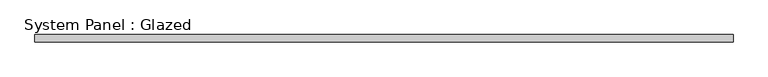
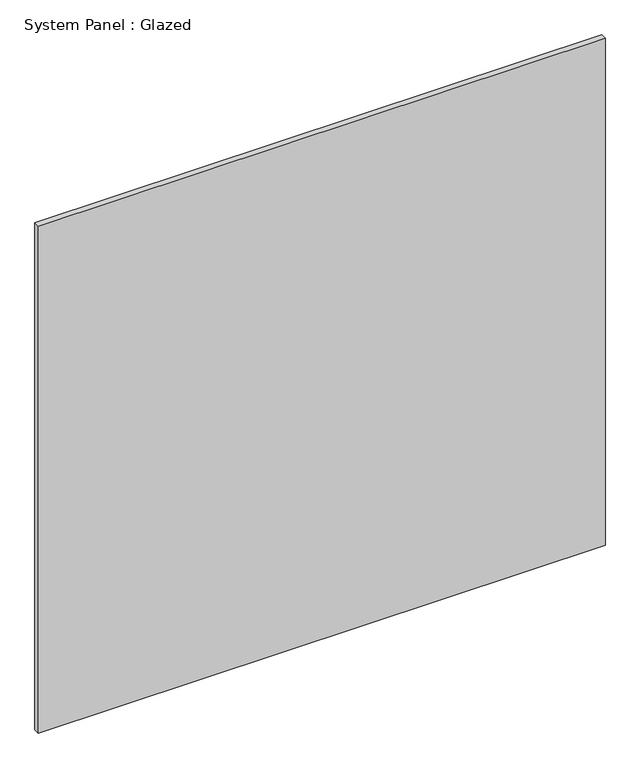
"""IFC4 building model written with IfcOpenShell, lengths in millimetres: plate geometry, System Panel : Glazed."""

from ifc_helpers import new_model, si_unit, origin, origin_with_axes, place, context, project, spatial, polyline, outline, extrude, source, transform, mapped, element, save


def system_panel_glazed_0b5a89bb(model_context):
    return source(origin(), model_context, "Body", "SweptSolid", [
        extrude(outline(polyline([(1222.996271, 19.05), (-1222.996271, 19.05), (-1222.996271, 44.45), (1222.996271, 44.45), (1222.996271, 19.05)])), origin_with_axes(), (0.0, 0.0, 1.0), 2311.4),
    ])


if __name__ == "__main__":
    model = new_model("IFC4")
    model_context = context("Model", 3, world=origin())
    ifc_project = project(units=[si_unit("LENGTHUNIT", "METRE", prefix="MILLI")], contexts=[model_context])
    site = spatial("IfcSite", under=ifc_project)
    building = spatial("IfcBuilding", under=site)
    placement = place(None, origin())
    system_panel_glazed_shape = system_panel_glazed_0b5a89bb(model_context)
    element("IfcPlate", 1, ObjectType="System Panel : Glazed", at=placement, inside=building, context=model_context, shape_type="MappedRepresentation", body=[
        mapped(system_panel_glazed_shape, transform((0.0, 0.0, 0.0), x_axis=(1.0, 0.0, 0.0), y_axis=(0.0, 1.0, 0.0), z_axis=(0.0, 0.0, 1.0))),
    ])
    save(model, "model.ifc")

# Revit data of these elements
# Type "System Panel : Glazed"
#   Construction Type Id = "GSP4R"
#   Analytic Construction = "1/8 in Pilkington single glazing"
#   Visual Light Transmittance = 0.9
#   Solar Heat Gain Coefficient = 0.86
#   Heat Transfer Coefficient (U) = 1.18115 BTU/(h·ft²·°F)
# Element 1 (IfcPlate, "System Panel : Glazed")
#   Materials on its faces: "Glass"
# Materials
#   "Glass": class "Glass", colour RGB 0 128 192, transparency 0.75, Description = "Soda Lime Glass", Cost = 0
